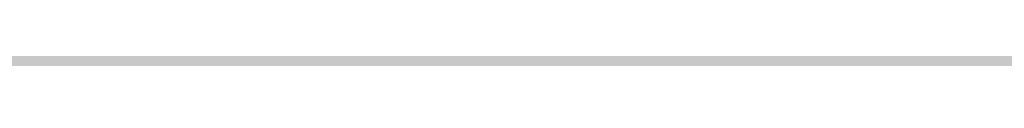
# Model space of a CAD drawing. Units: millimetres. Extents: x 0 to 2267, y 0 to 1823.
# Tile 97 of 256: x 1600.369 to 1605.705, y 1227.255 to 1227.263. Entities that reach past the tile are written whole.
import ezdxf

# ---------------------------------------------------------------- set-up
doc = ezdxf.new("R2010")
doc.units = ezdxf.units.MM
doc.header["$MEASUREMENT"] = 0
doc.layers.add('M-DIMS', color=2, linetype='Continuous', lineweight=25)
doc.layers.add('M-HATC', color=252, linetype='Continuous', lineweight=18)
doc.styles.get("Standard").update_dxf_attribs({"font": 'arial.ttf'})
doc.dimstyles.get("Standard").update_dxf_attribs({"dimtxt": 7, "dimasz": 4, "dimexe": 0.18, "dimexo": 0.0625, "dimgap": 0.09, "dimtad": 0, "dimdec": 0, "dimzin": 0, "dimdsep": 46, "dimtxsty": 'Standard', "dimcen": 0.09, "dimadec": 0, "dimazin": 0, "dimtfac": 1, "dimtdec": 0, "dimtofl": 0, "dimtmove": 0, "dimatfit": 3, "dimfxl": 1, "dimtolj": 1, "dimtzin": 0, "dimarcsym": 0})

# ---------------------------------------------------------------- blocks, each defined once
blk = doc.blocks.new('*D19')
at = {"layer": 'Defpoints', "color": 0, "transparency": 16777216}
for p in [(1605.3399, 1483.3044), (1445.5291, 1333.8851)]:
    blk.add_point(p, dxfattribs=at)
at = {"layer": 'M-DIMS', "color": 0, "lineweight": -2, "transparency": 16777216}
for p, q in [((1605.3399, 1483.2144), (1605.3399, 1483.3944)), ((1605.2499, 1483.3044), (1605.4299, 1483.3044)), ((1366.3244, 1259.8306), (1442.6072, 1331.1532))]:
    blk.add_line(p, q, dxfattribs=at)
at = {"layer": 'M-DIMS', "color": 0, "transparency": 16777216}
blk.add_solid([(1442.1519, 1331.6402), (1443.0625, 1330.6663), (1445.5291, 1333.8851)], dxfattribs=at)
at = {"layer": 'M-DIMS', "color": 0, "transparency": 16777216, "insert": (1349.6425, 1244.2335), "char_height": 7, "attachment_point": 5, "rotation": 43.0753}
blk.add_mtext('\\A1;2X R218.8', dxfattribs=at)

msp = doc.modelspace()

# ---------------------------------------------------------------- hatches: boundary and pattern name
at = {"layer": 'M-HATC'}
h = msp.add_hatch(color=256, dxfattribs=at)
h.dxf.hatch_style = 1
h.paths.add_polyline_path([(2055.771, 1603.062), (1381.0868, 1603.062), (1381.0868, 1598.062), (2055.771, 1598.062)])
h.paths.add_polyline_path([(2055.771, 1598.062), (1381.0868, 1598.062), (1381.0868, 1593.062), (2055.771, 1593.062)])
h.paths.add_polyline_path([(2051.3074, 1536.7609), (1385.5504, 1536.7609), (1385.5504, 1526.7609), (1387.5504, 1526.7609), (1388.5366, 1525.0528), (1385.3319, 1521.2335), (1385.3319, 1521.2226), (2050.2542, 1522.7491), (2048.3212, 1525.0528), (2049.3074, 1526.7609), (2051.3074, 1526.7609)])
edge = h.paths.add_edge_path()
edge.add_arc((1847.5345, 1379.1492), 135, 222.603061, 222.890851, ccw=False)
edge.add_line((1748.1663, 1287.7656), (1683.0921, 1287.7656))
edge.add_arc((1583.7239, 1379.1492), 135, 317.109149, 317.396939, ccw=False)
edge.add_arc((1678.9686, 1290.6707), 5, 222.8909, 317.1091, ccw=False)
edge.add_arc((1774.2133, 1379.1492), 135, 222.603061, 222.890851, ccw=False)
edge.add_line((1674.8451, 1287.7656), (1609.7709, 1287.7656))
edge.add_arc((1510.4027, 1379.1492), 135, 317.109149, 317.396939, ccw=False)
edge.add_arc((1605.6474, 1290.6707), 5, 222.8909, 317.1091, ccw=False)
edge.add_arc((1700.8921, 1379.1492), 135, 222.603061, 222.890851, ccw=False)
edge.add_line((1601.5239, 1287.7656), (1536.4497, 1287.7656))
edge.add_arc((1437.0815, 1379.1492), 135, 317.109149, 317.396939, ccw=False)
edge.add_arc((1532.3262, 1290.6707), 5, 222.8909, 317.1091, ccw=False)
edge.add_arc((1627.5709, 1379.1492), 135, 222.603061, 222.890851, ccw=False)
edge.add_line((1528.2027, 1287.7656), (1505.9289, 1287.7656))
edge.add_spline(control_points=[(1505.9289, 1287.7656), (1504.2622, 1287.7656), (1504.2622, 1282.7656), (1505.9289, 1282.7656)], knot_values=[0, 0, 0, 0, 5, 5, 5, 5], degree=3, periodic=0)
edge.add_line((1505.9289, 1282.7656), (1930.9289, 1282.7656))
edge.add_spline(control_points=[(1930.9289, 1282.7656), (1932.5956, 1282.7656), (1932.5956, 1287.7656), (1930.9289, 1287.7656)], knot_values=[0, 0, 0, 0, 5, 5, 5, 5], degree=3, periodic=0)
edge.add_line((1930.9289, 1287.7656), (1903.0557, 1287.7656))
edge.add_arc((1803.6875, 1379.1492), 135, 317.109149, 317.396939, ccw=False)
edge.add_arc((1898.9322, 1290.6707), 5, 222.8909, 317.1091, ccw=False)
edge.add_arc((1994.1769, 1379.1492), 135, 222.603061, 222.890851, ccw=False)
edge.add_line((1894.8087, 1287.7656), (1829.7345, 1287.7656))
edge.add_arc((1730.3663, 1379.1492), 135, 317.109149, 317.396939, ccw=False)
edge.add_arc((1825.611, 1290.6707), 5, 222.8909, 317.1091, ccw=False)
edge.add_arc((1920.8557, 1379.1492), 135, 222.603061, 222.890851, ccw=False)
edge.add_line((1821.4875, 1287.7656), (1756.4133, 1287.7656))
edge.add_arc((1657.0451, 1379.1492), 135, 317.109149, 317.396939, ccw=False)
edge.add_arc((1752.2898, 1290.6707), 5, 222.8909, 317.1091, ccw=False)
edge = h.paths.add_edge_path()
edge.add_spline(control_points=[(1843.4289, 1227.2475), (1845.0956, 1227.2475), (1845.0956, 1232.2475), (1843.4289, 1232.2475)], knot_values=[0, 0, 0, 0, 5, 5, 5, 5], degree=3, periodic=0)
edge.add_line((1843.4289, 1232.2475), (1593.4289, 1232.2475))
edge.add_spline(control_points=[(1593.4289, 1232.2475), (1591.7622, 1232.2475), (1591.7622, 1227.2475), (1593.4289, 1227.2475)], knot_values=[0, 0, 0, 0, 5, 5, 5, 5], degree=3, periodic=0)
edge.add_line((1593.4289, 1227.2475), (1843.4289, 1227.2475))
h.paths.add_polyline_path([(1905.9289, 1127.4171), (1530.9289, 1127.4171, 0.414214), (1520.9289, 1117.4171), (1530.9289, 1117.4171), (1915.9289, 1117.4171, 0.414214)])
edge = h.paths.add_edge_path()
edge.add_arc((1397.0858, 1498.4078), 12.7299, 90.78215, 190.87871, ccw=False)
edge.add_line((1396.912, 1511.1365), (1428.0097, 1511.3488))
edge.add_line((1428.0097, 1511.3488), (1433.0097, 1511.3488))
edge.add_line((1433.0097, 1511.3488), (1434.439, 1511.3488))
edge.add_arc((1419.474, 1498.0804), 20, 41.561, 74.08211)
edge.add_line((1424.9592, 1517.3135), (1399.9351, 1517.2561))
edge.add_spline(control_points=[(1399.9307, 1517.2561), (1399.884, 1517.2131), (1399.8328, 1517.1689), (1399.7774, 1517.1236)], knot_values=[11.567499, 11.567499, 11.567499, 11.567499, 11.814249, 11.814249, 11.814249, 11.814249], degree=3, periodic=0)
edge.add_spline(control_points=[(1399.6328, 1517.0099), (1399.5831, 1516.9721), (1399.5307, 1516.9338), (1399.4759, 1516.8947)], knot_values=[11.167718, 11.167718, 11.167718, 11.167718, 11.365188, 11.365188, 11.365188, 11.365188], degree=3, periodic=0)
edge.add_spline(control_points=[(1399.3398, 1516.8001), (1399.1514, 1516.6719), (1398.9384, 1516.5377), (1398.704, 1516.3994)], knot_values=[10.376405, 10.376405, 10.376405, 10.376405, 11.00994, 11.00994, 11.00994, 11.00994], degree=3, periodic=0)
edge.add_spline(control_points=[(1398.6572, 1516.3719), (1398.5789, 1516.326), (1398.4983, 1516.2797), (1398.4155, 1516.2331)], knot_values=[10.125175, 10.125175, 10.125175, 10.125175, 10.334406, 10.334406, 10.334406, 10.334406], degree=3, periodic=0)
edge.add_spline(control_points=[(1398.2642, 1516.1487), (1398.196, 1516.1111), (1398.1263, 1516.0732), (1398.0555, 1516.0351)], knot_values=[9.832246, 9.832246, 9.832246, 9.832246, 9.999658, 9.999658, 9.999658, 9.999658], degree=3, periodic=0)
edge.add_spline(control_points=[(1397.9987, 1516.0048), (1397.7312, 1515.8621), (1397.446, 1515.7171), (1397.1466, 1515.5714)], knot_values=[9.161808, 9.161808, 9.161808, 9.161808, 9.787769, 9.787769, 9.787769, 9.787769], degree=3, periodic=0)
edge.add_spline(control_points=[(1397.1466, 1515.5714), (1396.8418, 1515.423), (1396.5222, 1515.274), (1396.1914, 1515.1262)], knot_values=[8.524455, 8.524455, 8.524455, 8.524455, 9.161808, 9.161808, 9.161808, 9.161808], degree=3, periodic=0)
edge.add_spline(control_points=[(1396.0777, 1515.0756), (1395.9854, 1515.0348), (1395.8922, 1514.994), (1395.7983, 1514.9534)], knot_values=[8.275193, 8.275193, 8.275193, 8.275193, 8.451726, 8.451726, 8.451726, 8.451726], degree=3, periodic=0)
edge.add_spline(control_points=[(1395.6018, 1514.8691), (1395.4997, 1514.8257), (1395.3968, 1514.7824), (1395.2932, 1514.7394)], knot_values=[7.962917, 7.962917, 7.962917, 7.962917, 8.152764, 8.152764, 8.152764, 8.152764], degree=3, periodic=0)
edge.add_spline(control_points=[(1395.2116, 1514.7057), (1394.8278, 1514.5475), (1394.4345, 1514.3929), (1394.0364, 1514.2442)], knot_values=[7.21254, 7.21254, 7.21254, 7.21254, 7.913148, 7.913148, 7.913148, 7.913148], degree=3, periodic=0)
edge.add_spline(control_points=[(1394.0364, 1514.2442), (1393.7076, 1514.1214), (1393.3754, 1514.0027), (1393.0427, 1513.8895)], knot_values=[6.633733, 6.633733, 6.633733, 6.633733, 7.21254, 7.21254, 7.21254, 7.21254], degree=3, periodic=0)
edge.add_spline(control_points=[(1392.8214, 1513.815), (1392.7198, 1513.7812), (1392.6181, 1513.7479), (1392.5166, 1513.7152)], knot_values=[6.328796, 6.328796, 6.328796, 6.328796, 6.505493, 6.505493, 6.505493, 6.505493], degree=3, periodic=0)
edge.add_spline(control_points=[(1392.5166, 1513.7152), (1392.3187, 1513.6515), (1392.1212, 1513.59), (1391.9244, 1513.531)], knot_values=[5.984605, 5.984605, 5.984605, 5.984605, 6.328796, 6.328796, 6.328796, 6.328796], degree=3, periodic=0)
edge.add_spline(control_points=[(1391.7915, 1513.4915), (1391.3122, 1513.3501), (1390.8384, 1513.2239), (1390.3784, 1513.1171)], knot_values=[5.066697, 5.066697, 5.066697, 5.066697, 5.907055, 5.907055, 5.907055, 5.907055], degree=3, periodic=0)
edge.add_spline(control_points=[(1390.3784, 1513.1171), (1390.1797, 1513.071), (1389.9836, 1513.0284), (1389.7907, 1512.9899)], knot_values=[4.70367, 4.70367, 4.70367, 4.70367, 5.066695, 5.066695, 5.066695, 5.066695], degree=3, periodic=0)
edge.add_spline(control_points=[(1389.422, 1512.9204), (1389.2459, 1512.8892), (1389.0729, 1512.8617), (1388.9036, 1512.8381)], knot_values=[4.130571, 4.130571, 4.130571, 4.130571, 4.469816, 4.469816, 4.469816, 4.469816], degree=3, periodic=0)
edge.add_spline(control_points=[(1388.9036, 1512.8381), (1388.591, 1512.7946), (1388.2911, 1512.7644), (1388.0071, 1512.7494)], knot_values=[3.504031, 3.504031, 3.504031, 3.504031, 4.130571, 4.130571, 4.130571, 4.130571], degree=3, periodic=0)
edge.add_spline(control_points=[(1387.9356, 1512.7459), (1387.8538, 1512.7423), (1387.7733, 1512.74), (1387.6944, 1512.739)], knot_values=[3.268866, 3.268866, 3.268866, 3.268866, 3.451164, 3.451164, 3.451164, 3.451164], degree=3, periodic=0)
edge.add_spline(control_points=[(1387.3351, 1512.7443), (1387.2076, 1512.7499), (1387.0847, 1512.7597), (1386.967, 1512.7739)], knot_values=[2.670686, 2.670686, 2.670686, 2.670686, 2.984, 2.984, 2.984, 2.984], degree=3, periodic=0)
edge.add_spline(control_points=[(1386.8327, 1512.7922), (1386.8209, 1512.7941), (1386.8092, 1512.7959), (1386.7975, 1512.7979)], knot_values=[2.516981, 2.516981, 2.516981, 2.516981, 2.549528, 2.549528, 2.549528, 2.549528], degree=3, periodic=0)
edge.add_spline(control_points=[(1386.4526, 1512.8735), (1386.4257, 1512.881), (1386.3993, 1512.889), (1386.3733, 1512.8972)], knot_values=[2.095869, 2.095869, 2.095869, 2.095869, 2.17941, 2.17941, 2.17941, 2.17941], degree=3, periodic=0)
edge.add_spline(control_points=[(1386.0691, 1513.0189), (1386.0634, 1513.0217), (1386.0577, 1513.0246), (1386.052, 1513.0275)], knot_values=[1.72453, 1.72453, 1.72453, 1.72453, 1.745933, 1.745933, 1.745933, 1.745933], degree=3, periodic=0)
edge.add_arc((1399.474, 1498.0804), 20, 131.82432, 180)
edge.add_arc((1630.3336, 1505.5484), 250.9708, 181.705176, 236.427975)
edge.add_arc((1605.3399, 1483.3044), 218.7822, 238.660829, 243.34961)
edge.add_arc((1647.0911, 1510.3592), 262.8986, 183.129836, 237.853442, ccw=False)
h.paths.add_polyline_path([(1406.5369, 1391.9644, 0.149382), (1491.5506, 1296.4418, -0.129517)], flags=17)
edge = h.paths.add_edge_path()
edge.add_arc((2037.3838, 1498.0804), 20, 0, 48.26587)
edge.add_spline(control_points=[(2050.6973, 1513.0052), (2050.6512, 1512.9847), (2050.6034, 1512.9655), (2050.5539, 1512.9477)], knot_values=[1.835652, 1.835652, 1.835652, 1.835652, 2.000781, 2.000781, 2.000781, 2.000781], degree=3, periodic=0)
edge.add_spline(control_points=[(2050.4616, 1512.9166), (2050.479, 1512.9221), (2050.4963, 1512.9277), (2050.5133, 1512.9335)], knot_values=[2.045477, 2.045477, 2.045477, 2.045477, 2.101389, 2.101389, 2.101389, 2.101389], degree=3, periodic=0)
edge.add_spline(control_points=[(2050.129, 1512.8342), (2050.1984, 1512.8473), (2050.2657, 1512.8623), (2050.3308, 1512.8792)], knot_values=[2.237629, 2.237629, 2.237629, 2.237629, 2.435841, 2.435841, 2.435841, 2.435841], degree=3, periodic=0)
edge.add_spline(control_points=[(2050.0946, 1512.8278), (2050.1061, 1512.8299), (2050.1176, 1512.832), (2050.129, 1512.8342)], knot_values=[2.435841, 2.435841, 2.435841, 2.435841, 2.468321, 2.468321, 2.468321, 2.468321], degree=3, periodic=0)
edge.add_spline(control_points=[(2049.7843, 1512.7851), (2049.8552, 1512.7922), (2049.9243, 1512.8008), (2049.9917, 1512.8109)], knot_values=[2.563852, 2.563852, 2.563852, 2.563852, 2.748541, 2.748541, 2.748541, 2.748541], degree=3, periodic=0)
edge.add_spline(control_points=[(2049.4052, 1512.7617), (2049.5364, 1512.7653), (2049.6629, 1512.773), (2049.7843, 1512.7851)], knot_values=[2.748541, 2.748541, 2.748541, 2.748541, 3.064882, 3.064882, 3.064882, 3.064882], degree=3, periodic=0)
edge.add_spline(control_points=[(2049.1698, 1512.7597), (2049.2336, 1512.7591), (2049.2965, 1512.7594), (2049.3584, 1512.7606)], knot_values=[3.102309, 3.102309, 3.102309, 3.102309, 3.2503, 3.2503, 3.2503, 3.2503], degree=3, periodic=0)
edge.add_spline(control_points=[(2048.8573, 1512.7691), (2048.9638, 1512.7638), (2049.068, 1512.7606), (2049.1698, 1512.7597)], knot_values=[3.2503, 3.2503, 3.2503, 3.2503, 3.486069, 3.486069, 3.486069, 3.486069], degree=3, periodic=0)
edge.add_spline(control_points=[(2048.6924, 1512.7789), (2048.3729, 1512.8009), (2048.0345, 1512.8411), (2047.6817, 1512.897)], knot_values=[3.606429, 3.606429, 3.606429, 3.606429, 4.2989, 4.2989, 4.2989, 4.2989], degree=3, periodic=0)
edge.add_spline(control_points=[(2047.6817, 1512.897), (2047.5458, 1512.9185), (2047.4077, 1512.9424), (2047.2678, 1512.9685)], knot_values=[4.2989, 4.2989, 4.2989, 4.2989, 4.565769, 4.565769, 4.565769, 4.565769], degree=3, periodic=0)
edge.add_spline(control_points=[(2047.2678, 1512.9685), (2047.1449, 1512.9914), (2047.0207, 1513.016), (2046.8951, 1513.0422)], knot_values=[4.565769, 4.565769, 4.565769, 4.565769, 4.799971, 4.799971, 4.799971, 4.799971], degree=3, periodic=0)
edge.add_spline(control_points=[(2046.8951, 1513.0422), (2046.5286, 1513.1188), (2046.1513, 1513.209), (2045.7676, 1513.3107)], knot_values=[4.799971, 4.799971, 4.799971, 4.799971, 5.483718, 5.483718, 5.483718, 5.483718], degree=3, periodic=0)
edge.add_spline(control_points=[(2045.7676, 1513.3107), (2045.3724, 1513.4154), (2044.9704, 1513.5322), (2044.5662, 1513.6588)], knot_values=[5.483718, 5.483718, 5.483718, 5.483718, 6.187866, 6.187866, 6.187866, 6.187866], degree=3, periodic=0)
edge.add_spline(control_points=[(2044.5662, 1513.6588), (2044.4149, 1513.7061), (2044.2633, 1513.7549), (2044.1116, 1513.8048)], knot_values=[6.187866, 6.187866, 6.187866, 6.187866, 6.451551, 6.451551, 6.451551, 6.451551], degree=3, periodic=0)
edge.add_spline(control_points=[(2044.1116, 1513.8048), (2043.9967, 1513.8427), (2043.8817, 1513.8813), (2043.7668, 1513.9205)], knot_values=[6.451551, 6.451551, 6.451551, 6.451551, 6.651434, 6.651434, 6.651434, 6.651434], degree=3, periodic=0)
edge.add_spline(control_points=[(2043.7668, 1513.9205), (2043.3716, 1514.0554), (2042.9774, 1514.1979), (2042.5886, 1514.3458)], knot_values=[6.651434, 6.651434, 6.651434, 6.651434, 7.338879, 7.338879, 7.338879, 7.338879], degree=3, periodic=0)
edge.add_spline(control_points=[(2042.5886, 1514.3458), (2042.1643, 1514.5071), (2041.7465, 1514.6749), (2041.3409, 1514.846)], knot_values=[7.338879, 7.338879, 7.338879, 7.338879, 8.089209, 8.089209, 8.089209, 8.089209], degree=3, periodic=0)
edge.add_spline(control_points=[(2041.3409, 1514.846), (2041.1028, 1514.9465), (2040.869, 1515.0481), (2040.6405, 1515.1502)], knot_values=[8.089209, 8.089209, 8.089209, 8.089209, 8.529587, 8.529587, 8.529587, 8.529587], degree=3, periodic=0)
edge.add_spline(control_points=[(2040.51, 1515.2089), (2040.0824, 1515.4022), (2039.6747, 1515.5971), (2039.295, 1515.7894)], knot_values=[8.613818, 8.613818, 8.613818, 8.613818, 9.44571, 9.44571, 9.44571, 9.44571], degree=3, periodic=0)
edge.add_spline(control_points=[(2039.295, 1515.7894), (2039.0618, 1515.9075), (2038.8391, 1516.0246), (2038.6288, 1516.1398)], knot_values=[9.44571, 9.44571, 9.44571, 9.44571, 9.956404, 9.956404, 9.956404, 9.956404], degree=3, periodic=0)
edge.add_spline(control_points=[(2038.6288, 1516.1398), (2038.5187, 1516.2001), (2038.4121, 1516.2598), (2038.309, 1516.3189)], knot_values=[9.956404, 9.956404, 9.956404, 9.956404, 10.223542, 10.223542, 10.223542, 10.223542], degree=3, periodic=0)
edge.add_spline(control_points=[(2038.309, 1516.3189), (2038.2138, 1516.3735), (2038.1216, 1516.4276), (2038.0328, 1516.481)], knot_values=[10.223542, 10.223542, 10.223542, 10.223542, 10.47051, 10.47051, 10.47051, 10.47051], degree=3, periodic=0)
edge.add_spline(control_points=[(2038.0328, 1516.481), (2037.7855, 1516.6296), (2037.5639, 1516.773), (2037.3722, 1516.909)], knot_values=[10.47051, 10.47051, 10.47051, 10.47051, 11.15767, 11.15767, 11.15767, 11.15767], degree=3, periodic=0)
edge.add_spline(control_points=[(2037.3722, 1516.909), (2037.2789, 1516.9752), (2037.1927, 1517.0396), (2037.1142, 1517.102)], knot_values=[11.15767, 11.15767, 11.15767, 11.15767, 11.49227, 11.49227, 11.49227, 11.49227], degree=3, periodic=0)
edge.add_spline(control_points=[(2036.8564, 1517.3259), (2036.9148, 1517.2692), (2036.9814, 1517.2103), (2037.0557, 1517.1492)], knot_values=[11.577341, 11.577341, 11.577341, 11.577341, 11.91035, 11.91035, 11.91035, 11.91035], degree=3, periodic=0)
edge.add_spline(control_points=[(2036.8074, 1517.3748), (2036.823, 1517.3587), (2036.8393, 1517.3424), (2036.8564, 1517.3259)], knot_values=[11.91035, 11.91035, 11.91035, 11.91035, 12.007402, 12.007402, 12.007402, 12.007402], degree=3, periodic=0)
edge.add_spline(control_points=[(2036.7017, 1517.494), (2036.7104, 1517.483), (2036.7196, 1517.4719), (2036.7291, 1517.4606)], knot_values=[12.184155, 12.184155, 12.184155, 12.184155, 12.255409, 12.255409, 12.255409, 12.255409], degree=3, periodic=0)
edge.add_spline(control_points=[(2036.6159, 1517.6205), (2036.62, 1517.613), (2036.6243, 1517.6055), (2036.6289, 1517.5979)], knot_values=[12.487913, 12.487913, 12.487913, 12.487913, 12.541035, 12.541035, 12.541035, 12.541035], degree=3, periodic=0)
edge.add_spline(control_points=[(2036.5635, 1517.786), (2036.5637, 1517.7794), (2036.5642, 1517.7726), (2036.565, 1517.7658)], knot_values=[12.911761, 12.911761, 12.911761, 12.911761, 12.968286, 12.968286, 12.968286, 12.968286], degree=3, periodic=0)
edge.add_spline(control_points=[(2036.6166, 1517.9304), (2036.6125, 1517.9259), (2036.6086, 1517.9212), (2036.6049, 1517.9165)], knot_values=[13.382527, 13.382527, 13.382527, 13.382527, 13.433791, 13.433791, 13.433791, 13.433791], degree=3, periodic=0)
edge.add_spline(control_points=[(2036.749, 1518.017), (2036.7361, 1518.0116), (2036.7239, 1518.006), (2036.7124, 1518.0002)], knot_values=[13.726299, 13.726299, 13.726299, 13.726299, 13.809928, 13.809928, 13.809928, 13.809928], degree=3, periodic=0)
edge.add_spline(control_points=[(2036.8604, 1518.0528), (2036.8386, 1518.0474), (2036.8181, 1518.0416), (2036.7988, 1518.0353)], knot_values=[13.910887, 13.910887, 13.910887, 13.910887, 14.02153, 14.02153, 14.02153, 14.02153], degree=3, periodic=0)
edge.add_line((2036.9639, 1518.0804), (2032.3838, 1518.0804))
edge.add_line((2032.3838, 1518.0804), (2027.3838, 1518.0804))
edge.add_line((2027.3838, 1518.0804), (2022.3838, 1518.0804))
edge.add_line((2022.3838, 1518.0804), (2017.3838, 1518.0804))
edge.add_arc((2017.3838, 1498.0804), 20, 90, 138.439)
edge.add_line((2002.4188, 1511.3488), (2003.8481, 1511.3488))
edge.add_line((2003.8481, 1511.3488), (2008.8481, 1511.3488))
edge.add_line((2008.8481, 1511.3488), (2039.772, 1511.1377))
edge.add_arc((2039.772, 1498.4078), 12.7299, -10.87871, 90, ccw=False)
edge.add_arc((1789.7668, 1510.3592), 262.8986, 302.146558, 356.870164, ccw=False)
edge.add_arc((1831.5179, 1483.3044), 218.7822, 296.65039, 301.339171)
edge.add_arc((1806.5242, 1505.5484), 250.9708, 303.572025, 358.294824)
h.paths.add_polyline_path([(2030.321, 1391.9644, -0.129517), (1945.3072, 1296.4418, 0.149382)], flags=17)
edge = h.paths.add_edge_path()
edge.add_spline(control_points=[(2037.2464, 1518.0821), (2037.2898, 1518.081), (2037.3355, 1518.0804), (2037.3838, 1518.0804)], knot_values=[0.000012, 0.000012, 0.000012, 0.000012, 0.144754, 0.144754, 0.144754, 0.144754], degree=3, periodic=0)
edge.add_line((2037.3357, 1518.0804), (2037.0096, 1518.0804))
edge.add_spline(control_points=[(2037.0096, 1518.0804), (2036.9822, 1518.0768), (2036.956, 1518.0727), (2036.9312, 1518.0681)], knot_values=[14.13465, 14.13465, 14.13465, 14.13465, 14.247197, 14.247197, 14.247197, 14.247197], degree=3, periodic=0)
edge.add_spline(control_points=[(2036.9312, 1518.0681), (2036.9276, 1518.0674), (2036.9241, 1518.0667), (2036.9205, 1518.0661)], knot_values=[14.118315, 14.118315, 14.118315, 14.118315, 14.13465, 14.13465, 14.13465, 14.13465], degree=3, periodic=0)
edge.add_spline(control_points=[(2036.9205, 1518.0661), (2036.9118, 1518.0644), (2036.9032, 1518.0626), (2036.8948, 1518.0608)], knot_values=[14.078086, 14.078086, 14.078086, 14.078086, 14.118315, 14.118315, 14.118315, 14.118315], degree=3, periodic=0)
edge.add_spline(control_points=[(2036.8948, 1518.0608), (2036.883, 1518.0583), (2036.8716, 1518.0556), (2036.8604, 1518.0528)], knot_values=[14.02153, 14.02153, 14.02153, 14.02153, 14.078086, 14.078086, 14.078086, 14.078086], degree=3, periodic=0)
edge.add_spline(control_points=[(2036.8604, 1518.0528), (2036.8386, 1518.0474), (2036.8181, 1518.0416), (2036.7988, 1518.0353)], knot_values=[13.910887, 13.910887, 13.910887, 13.910887, 14.02153, 14.02153, 14.02153, 14.02153], degree=3, periodic=0)
edge.add_spline(control_points=[(2036.7988, 1518.0353), (2036.7981, 1518.035), (2036.7974, 1518.0348), (2036.7967, 1518.0346)], knot_values=[13.906906, 13.906906, 13.906906, 13.906906, 13.910887, 13.910887, 13.910887, 13.910887], degree=3, periodic=0)
edge.add_spline(control_points=[(2036.7967, 1518.0346), (2036.7882, 1518.0318), (2036.7799, 1518.0289), (2036.7719, 1518.0259)], knot_values=[13.857826, 13.857826, 13.857826, 13.857826, 13.906906, 13.906906, 13.906906, 13.906906], degree=3, periodic=0)
edge.add_spline(control_points=[(2036.7719, 1518.0259), (2036.764, 1518.023), (2036.7564, 1518.02), (2036.749, 1518.017)], knot_values=[13.809928, 13.809928, 13.809928, 13.809928, 13.857826, 13.857826, 13.857826, 13.857826], degree=3, periodic=0)
edge.add_spline(control_points=[(2036.749, 1518.017), (2036.7361, 1518.0116), (2036.7239, 1518.006), (2036.7124, 1518.0002)], knot_values=[13.726299, 13.726299, 13.726299, 13.726299, 13.809928, 13.809928, 13.809928, 13.809928], degree=3, periodic=0)
edge.add_spline(control_points=[(2036.7124, 1518.0002), (2036.7121, 1518), (2036.7118, 1517.9999), (2036.7115, 1517.9997)], knot_values=[13.723993, 13.723993, 13.723993, 13.723993, 13.726299, 13.726299, 13.726299, 13.726299], degree=3, periodic=0)
edge.add_spline(control_points=[(2036.7115, 1517.9997), (2036.7063, 1517.9971), (2036.7013, 1517.9944), (2036.6965, 1517.9917)], knot_values=[13.686536, 13.686536, 13.686536, 13.686536, 13.723993, 13.723993, 13.723993, 13.723993], degree=3, periodic=0)
edge.add_spline(control_points=[(2036.6965, 1517.9917), (2036.6919, 1517.9891), (2036.6874, 1517.9865), (2036.6831, 1517.9839)], knot_values=[13.651251, 13.651251, 13.651251, 13.651251, 13.686536, 13.686536, 13.686536, 13.686536], degree=3, periodic=0)
edge.add_spline(control_points=[(2036.6831, 1517.9839), (2036.6764, 1517.9798), (2036.67, 1517.9757), (2036.6639, 1517.9714)], knot_values=[13.596804, 13.596804, 13.596804, 13.596804, 13.651251, 13.651251, 13.651251, 13.651251], degree=3, periodic=0)
edge.add_spline(control_points=[(2036.6639, 1517.9714), (2036.6636, 1517.9712), (2036.6633, 1517.9709), (2036.6629, 1517.9707)], knot_values=[13.593956, 13.593956, 13.593956, 13.593956, 13.596804, 13.596804, 13.596804, 13.596804], degree=3, periodic=0)
edge.add_spline(control_points=[(2036.6629, 1517.9707), (2036.6603, 1517.9689), (2036.6577, 1517.967), (2036.6552, 1517.9651)], knot_values=[13.570322, 13.570322, 13.570322, 13.570322, 13.593956, 13.593956, 13.593956, 13.593956], degree=3, periodic=0)
edge.add_spline(control_points=[(2036.6552, 1517.9651), (2036.6525, 1517.9631), (2036.6499, 1517.9611), (2036.6474, 1517.9591)], knot_values=[13.545477, 13.545477, 13.545477, 13.545477, 13.570322, 13.570322, 13.570322, 13.570322], degree=3, periodic=0)
edge.add_spline(control_points=[(2036.6474, 1517.9591), (2036.6472, 1517.9589), (2036.6471, 1517.9588), (2036.6469, 1517.9587)], knot_values=[13.543931, 13.543931, 13.543931, 13.543931, 13.545477, 13.545477, 13.545477, 13.545477], degree=3, periodic=0)
edge.add_spline(control_points=[(2036.6469, 1517.9587), (2036.6412, 1517.9541), (2036.6358, 1517.9494), (2036.6307, 1517.9447)], knot_values=[13.488237, 13.488237, 13.488237, 13.488237, 13.543931, 13.543931, 13.543931, 13.543931], degree=3, periodic=0)
edge.add_spline(control_points=[(2036.6307, 1517.9447), (2036.6282, 1517.9423), (2036.6257, 1517.9399), (2036.6233, 1517.9374)], knot_values=[13.460307, 13.460307, 13.460307, 13.460307, 13.488237, 13.488237, 13.488237, 13.488237], degree=3, periodic=0)
edge.add_spline(control_points=[(2036.6233, 1517.9374), (2036.6215, 1517.9356), (2036.6198, 1517.9338), (2036.6181, 1517.932)], knot_values=[13.439712, 13.439712, 13.439712, 13.439712, 13.460307, 13.460307, 13.460307, 13.460307], degree=3, periodic=0)
edge.add_spline(control_points=[(2036.6181, 1517.932), (2036.6176, 1517.9315), (2036.6171, 1517.9309), (2036.6166, 1517.9304)], knot_values=[13.433791, 13.433791, 13.433791, 13.433791, 13.439712, 13.439712, 13.439712, 13.439712], degree=3, periodic=0)
edge.add_spline(control_points=[(2036.6166, 1517.9304), (2036.6125, 1517.9259), (2036.6086, 1517.9212), (2036.6049, 1517.9165)], knot_values=[13.382527, 13.382527, 13.382527, 13.382527, 13.433791, 13.433791, 13.433791, 13.433791], degree=3, periodic=0)
edge.add_spline(control_points=[(2036.6049, 1517.9165), (2036.6026, 1517.9135), (2036.6004, 1517.9104), (2036.5982, 1517.9074)], knot_values=[13.350017, 13.350017, 13.350017, 13.350017, 13.382527, 13.382527, 13.382527, 13.382527], degree=3, periodic=0)
edge.add_spline(control_points=[(2036.5982, 1517.9074), (2036.5972, 1517.9059), (2036.5962, 1517.9043), (2036.5952, 1517.9028)], knot_values=[13.333922, 13.333922, 13.333922, 13.333922, 13.350017, 13.350017, 13.350017, 13.350017], degree=3, periodic=0)
edge.add_spline(control_points=[(2036.5952, 1517.9028), (2036.5945, 1517.9018), (2036.5939, 1517.9009), (2036.5933, 1517.8999)], knot_values=[13.323828, 13.323828, 13.323828, 13.323828, 13.333922, 13.333922, 13.333922, 13.333922], degree=3, periodic=0)
edge.add_spline(control_points=[(2036.5933, 1517.8999), (2036.5905, 1517.8955), (2036.5879, 1517.8909), (2036.5855, 1517.8864)], knot_values=[13.277545, 13.277545, 13.277545, 13.277545, 13.323828, 13.323828, 13.323828, 13.323828], degree=3, periodic=0)
edge.add_spline(control_points=[(2036.5855, 1517.8864), (2036.5836, 1517.8827), (2036.5817, 1517.8789), (2036.5801, 1517.8751)], knot_values=[13.240119, 13.240119, 13.240119, 13.240119, 13.277545, 13.277545, 13.277545, 13.277545], degree=3, periodic=0)
edge.add_spline(control_points=[(2036.5801, 1517.8751), (2036.5795, 1517.8739), (2036.579, 1517.8727), (2036.5785, 1517.8715)], knot_values=[13.228211, 13.228211, 13.228211, 13.228211, 13.240119, 13.240119, 13.240119, 13.240119], degree=3, periodic=0)
edge.add_spline(control_points=[(2036.5785, 1517.8715), (2036.578, 1517.8702), (2036.5774, 1517.869), (2036.5769, 1517.8677)], knot_values=[13.215717, 13.215717, 13.215717, 13.215717, 13.228211, 13.228211, 13.228211, 13.228211], degree=3, periodic=0)
edge.add_spline(control_points=[(2036.5769, 1517.8677), (2036.5755, 1517.864), (2036.5741, 1517.8603), (2036.5729, 1517.8565)], knot_values=[13.179847, 13.179847, 13.179847, 13.179847, 13.215717, 13.215717, 13.215717, 13.215717], degree=3, periodic=0)
edge.add_spline(control_points=[(2036.5729, 1517.8565), (2036.5713, 1517.8515), (2036.5699, 1517.8464), (2036.5687, 1517.8413)], knot_values=[13.132017, 13.132017, 13.132017, 13.132017, 13.179847, 13.179847, 13.179847, 13.179847], degree=3, periodic=0)
edge.add_spline(control_points=[(2036.5687, 1517.8413), (2036.5684, 1517.8402), (2036.5682, 1517.8392), (2036.568, 1517.8382)], knot_values=[13.122482, 13.122482, 13.122482, 13.122482, 13.132017, 13.132017, 13.132017, 13.132017], degree=3, periodic=0)
edge.add_spline(control_points=[(2036.568, 1517.8382), (2036.5676, 1517.8363), (2036.5672, 1517.8345), (2036.5669, 1517.8327)], knot_values=[13.105592, 13.105592, 13.105592, 13.105592, 13.122482, 13.122482, 13.122482, 13.122482], degree=3, periodic=0)
edge.add_spline(control_points=[(2036.5669, 1517.8327), (2036.5662, 1517.8292), (2036.5657, 1517.8257), (2036.5652, 1517.8222)], knot_values=[13.074063, 13.074063, 13.074063, 13.074063, 13.105592, 13.105592, 13.105592, 13.105592], degree=3, periodic=0)
edge.add_spline(control_points=[(2036.5652, 1517.8222), (2036.5652, 1517.8222), (2036.5652, 1517.8222), (2036.5652, 1517.8222)], knot_values=[13.074043, 13.074043, 13.074043, 13.074043, 13.074063, 13.074063, 13.074063, 13.074063], degree=3, periodic=0)
edge.add_spline(control_points=[(2036.5652, 1517.8222), (2036.5644, 1517.8164), (2036.5639, 1517.8106), (2036.5636, 1517.8046)], knot_values=[13.021884, 13.021884, 13.021884, 13.021884, 13.074043, 13.074043, 13.074043, 13.074043], degree=3, periodic=0)
edge.add_spline(control_points=[(2036.5636, 1517.8046), (2036.5636, 1517.804), (2036.5636, 1517.8034), (2036.5635, 1517.8028)], knot_values=[13.01674, 13.01674, 13.01674, 13.01674, 13.021884, 13.021884, 13.021884, 13.021884], degree=3, periodic=0)
edge.add_spline(control_points=[(2036.5635, 1517.8028), (2036.5634, 1517.8005), (2036.5634, 1517.7982), (2036.5634, 1517.7958)], knot_values=[12.996438, 12.996438, 12.996438, 12.996438, 13.01674, 13.01674, 13.01674, 13.01674], degree=3, periodic=0)
edge.add_spline(control_points=[(2036.5634, 1517.7958), (2036.5633, 1517.7926), (2036.5634, 1517.7893), (2036.5635, 1517.786)], knot_values=[12.968286, 12.968286, 12.968286, 12.968286, 12.996438, 12.996438, 12.996438, 12.996438], degree=3, periodic=0)
edge.add_spline(control_points=[(2036.5635, 1517.786), (2036.5637, 1517.7794), (2036.5642, 1517.7726), (2036.565, 1517.7658)], knot_values=[12.911761, 12.911761, 12.911761, 12.911761, 12.968286, 12.968286, 12.968286, 12.968286], degree=3, periodic=0)
edge.add_spline(control_points=[(2036.565, 1517.7658), (2036.565, 1517.7657), (2036.565, 1517.7656), (2036.565, 1517.7656)], knot_values=[12.911017, 12.911017, 12.911017, 12.911017, 12.911761, 12.911761, 12.911761, 12.911761], degree=3, periodic=0)
edge.add_spline(control_points=[(2036.565, 1517.7656), (2036.5654, 1517.7625), (2036.5658, 1517.7593), (2036.5663, 1517.7562)], knot_values=[12.88528, 12.88528, 12.88528, 12.88528, 12.911017, 12.911017, 12.911017, 12.911017], degree=3, periodic=0)
edge.add_spline(control_points=[(2036.5663, 1517.7562), (2036.5667, 1517.7534), (2036.5672, 1517.7506), (2036.5677, 1517.7478)], knot_values=[12.862519, 12.862519, 12.862519, 12.862519, 12.88528, 12.88528, 12.88528, 12.88528], degree=3, periodic=0)
edge.add_spline(control_points=[(2036.5677, 1517.7478), (2036.5678, 1517.7474), (2036.5679, 1517.7469), (2036.568, 1517.7465)], knot_values=[12.858885, 12.858885, 12.858885, 12.858885, 12.862519, 12.862519, 12.862519, 12.862519], degree=3, periodic=0)
edge.add_spline(control_points=[(2036.568, 1517.7465), (2036.5692, 1517.7399), (2036.5707, 1517.7332), (2036.5724, 1517.7264)], knot_values=[12.8053, 12.8053, 12.8053, 12.8053, 12.858885, 12.858885, 12.858885, 12.858885], degree=3, periodic=0)
edge.add_spline(control_points=[(2036.5724, 1517.7264), (2036.5734, 1517.7226), (2036.5745, 1517.7187), (2036.5756, 1517.7149)], knot_values=[12.775176, 12.775176, 12.775176, 12.775176, 12.8053, 12.8053, 12.8053, 12.8053], degree=3, periodic=0)
edge.add_spline(control_points=[(2036.5756, 1517.7149), (2036.5763, 1517.7125), (2036.577, 1517.7102), (2036.5778, 1517.7078)], knot_values=[12.756759, 12.756759, 12.756759, 12.756759, 12.775176, 12.775176, 12.775176, 12.775176], degree=3, periodic=0)
edge.add_spline(control_points=[(2036.5778, 1517.7078), (2036.5781, 1517.7067), (2036.5784, 1517.7057), (2036.5787, 1517.7047)], knot_values=[12.748742, 12.748742, 12.748742, 12.748742, 12.756759, 12.756759, 12.756759, 12.756759], degree=3, periodic=0)
edge.add_spline(control_points=[(2036.5787, 1517.7047), (2036.5808, 1517.6983), (2036.5831, 1517.6919), (2036.5856, 1517.6854)], knot_values=[12.69959, 12.69959, 12.69959, 12.69959, 12.748742, 12.748742, 12.748742, 12.748742], degree=3, periodic=0)
edge.add_spline(control_points=[(2036.5856, 1517.6854), (2036.5876, 1517.68), (2036.5898, 1517.6746), (2036.5921, 1517.6692)], knot_values=[12.659038, 12.659038, 12.659038, 12.659038, 12.69959, 12.69959, 12.69959, 12.69959], degree=3, periodic=0)
edge.add_spline(control_points=[(2036.5921, 1517.6692), (2036.594, 1517.6648), (2036.5959, 1517.6605), (2036.5979, 1517.6561)], knot_values=[12.626806, 12.626806, 12.626806, 12.626806, 12.659038, 12.659038, 12.659038, 12.659038], degree=3, periodic=0)
edge.add_spline(control_points=[(2036.5979, 1517.6561), (2036.5984, 1517.6551), (2036.5989, 1517.6541), (2036.5993, 1517.6531)], knot_values=[12.619394, 12.619394, 12.619394, 12.619394, 12.626806, 12.626806, 12.626806, 12.626806], degree=3, periodic=0)
edge.add_spline(control_points=[(2036.5993, 1517.6531), (2036.6043, 1517.6424), (2036.6099, 1517.6315), (2036.6159, 1517.6205)], knot_values=[12.541039, 12.541039, 12.541039, 12.541039, 12.619394, 12.619394, 12.619394, 12.619394], degree=3, periodic=0)
edge.add_spline(control_points=[(2036.6159, 1517.6205), (2036.6159, 1517.6205), (2036.6159, 1517.6205), (2036.6159, 1517.6205)], knot_values=[12.541035, 12.541035, 12.541035, 12.541035, 12.541039, 12.541039, 12.541039, 12.541039], degree=3, periodic=0)
edge.add_spline(control_points=[(2036.6159, 1517.6205), (2036.62, 1517.613), (2036.6243, 1517.6055), (2036.6289, 1517.5979)], knot_values=[12.487913, 12.487913, 12.487913, 12.487913, 12.541035, 12.541035, 12.541035, 12.541035], degree=3, periodic=0)
edge.add_spline(control_points=[(2036.6289, 1517.5979), (2036.6326, 1517.5916), (2036.6365, 1517.5853), (2036.6406, 1517.5789)], knot_values=[12.443982, 12.443982, 12.443982, 12.443982, 12.487913, 12.487913, 12.487913, 12.487913], degree=3, periodic=0)
edge.add_spline(control_points=[(2036.6406, 1517.5789), (2036.6414, 1517.5776), (2036.6423, 1517.5763), (2036.6431, 1517.5749)], knot_values=[12.434996, 12.434996, 12.434996, 12.434996, 12.443982, 12.443982, 12.443982, 12.443982], degree=3, periodic=0)
edge.add_spline(control_points=[(2036.6431, 1517.5749), (2036.6531, 1517.5596), (2036.6639, 1517.5439), (2036.6756, 1517.528)], knot_values=[12.329647, 12.329647, 12.329647, 12.329647, 12.434996, 12.434996, 12.434996, 12.434996], degree=3, periodic=0)
edge.add_spline(control_points=[(2036.6756, 1517.528), (2036.6839, 1517.5168), (2036.6925, 1517.5055), (2036.7017, 1517.494)], knot_values=[12.255409, 12.255409, 12.255409, 12.255409, 12.329647, 12.329647, 12.329647, 12.329647], degree=3, periodic=0)
edge.add_spline(control_points=[(2036.7017, 1517.494), (2036.7104, 1517.483), (2036.7196, 1517.4719), (2036.7291, 1517.4606)], knot_values=[12.184155, 12.184155, 12.184155, 12.184155, 12.255409, 12.255409, 12.255409, 12.255409], degree=3, periodic=0)
edge.add_spline(control_points=[(2036.7291, 1517.4606), (2036.7436, 1517.4435), (2036.759, 1517.4262), (2036.7753, 1517.4085)], knot_values=[12.075961, 12.075961, 12.075961, 12.075961, 12.184155, 12.184155, 12.184155, 12.184155], degree=3, periodic=0)
edge.add_spline(control_points=[(2036.7753, 1517.4085), (2036.7763, 1517.4075), (2036.7773, 1517.4064), (2036.7783, 1517.4054)], knot_values=[12.069502, 12.069502, 12.069502, 12.069502, 12.075961, 12.075961, 12.075961, 12.075961], degree=3, periodic=0)
edge.add_spline(control_points=[(2036.7783, 1517.4054), (2036.7877, 1517.3953), (2036.7974, 1517.385), (2036.8074, 1517.3748)], knot_values=[12.007402, 12.007402, 12.007402, 12.007402, 12.069502, 12.069502, 12.069502, 12.069502], degree=3, periodic=0)
edge.add_spline(control_points=[(2036.8074, 1517.3748), (2036.823, 1517.3587), (2036.8393, 1517.3424), (2036.8564, 1517.3259)], knot_values=[11.91035, 11.91035, 11.91035, 11.91035, 12.007402, 12.007402, 12.007402, 12.007402], degree=3, periodic=0)
edge.add_spline(control_points=[(2036.8564, 1517.3259), (2036.9148, 1517.2692), (2036.9814, 1517.2103), (2037.0557, 1517.1492)], knot_values=[11.577341, 11.577341, 11.577341, 11.577341, 11.91035, 11.91035, 11.91035, 11.91035], degree=3, periodic=0)
edge.add_spline(control_points=[(2037.0557, 1517.1492), (2037.0747, 1517.1336), (2037.0942, 1517.1179), (2037.1142, 1517.102)], knot_values=[11.49227, 11.49227, 11.49227, 11.49227, 11.577341, 11.577341, 11.577341, 11.577341], degree=3, periodic=0)
edge.add_spline(control_points=[(2037.1142, 1517.102), (2037.1927, 1517.0396), (2037.2789, 1516.9752), (2037.3722, 1516.909)], knot_values=[11.15767, 11.15767, 11.15767, 11.15767, 11.49227, 11.49227, 11.49227, 11.49227], degree=3, periodic=0)
edge.add_spline(control_points=[(2037.3722, 1516.909), (2037.5639, 1516.773), (2037.7855, 1516.6296), (2038.0328, 1516.481)], knot_values=[10.47051, 10.47051, 10.47051, 10.47051, 11.15767, 11.15767, 11.15767, 11.15767], degree=3, periodic=0)
edge.add_spline(control_points=[(2038.0328, 1516.481), (2038.1216, 1516.4276), (2038.2138, 1516.3735), (2038.309, 1516.3189)], knot_values=[10.223542, 10.223542, 10.223542, 10.223542, 10.47051, 10.47051, 10.47051, 10.47051], degree=3, periodic=0)
edge.add_spline(control_points=[(2038.309, 1516.3189), (2038.4121, 1516.2598), (2038.5187, 1516.2001), (2038.6288, 1516.1398)], knot_values=[9.956404, 9.956404, 9.956404, 9.956404, 10.223542, 10.223542, 10.223542, 10.223542], degree=3, periodic=0)
edge.add_spline(control_points=[(2038.6288, 1516.1398), (2038.8391, 1516.0246), (2039.0618, 1515.9075), (2039.295, 1515.7894)], knot_values=[9.44571, 9.44571, 9.44571, 9.44571, 9.956404, 9.956404, 9.956404, 9.956404], degree=3, periodic=0)
edge.add_spline(control_points=[(2039.295, 1515.7894), (2039.6747, 1515.5971), (2040.0824, 1515.4022), (2040.51, 1515.2089)], knot_values=[8.613818, 8.613818, 8.613818, 8.613818, 9.44571, 9.44571, 9.44571, 9.44571], degree=3, periodic=0)
edge.add_spline(control_points=[(2040.51, 1515.2089), (2040.5533, 1515.1893), (2040.5968, 1515.1697), (2040.6405, 1515.1502)], knot_values=[8.529587, 8.529587, 8.529587, 8.529587, 8.613818, 8.613818, 8.613818, 8.613818], degree=3, periodic=0)
edge.add_spline(control_points=[(2040.6405, 1515.1502), (2040.869, 1515.0481), (2041.1028, 1514.9465), (2041.3409, 1514.846)], knot_values=[8.089209, 8.089209, 8.089209, 8.089209, 8.529587, 8.529587, 8.529587, 8.529587], degree=3, periodic=0)
edge.add_spline(control_points=[(2041.3409, 1514.846), (2041.7465, 1514.6749), (2042.1643, 1514.5071), (2042.5886, 1514.3458)], knot_values=[7.338879, 7.338879, 7.338879, 7.338879, 8.089209, 8.089209, 8.089209, 8.089209], degree=3, periodic=0)
edge.add_spline(control_points=[(2042.5886, 1514.3458), (2042.9774, 1514.1979), (2043.3716, 1514.0554), (2043.7668, 1513.9205)], knot_values=[6.651434, 6.651434, 6.651434, 6.651434, 7.338879, 7.338879, 7.338879, 7.338879], degree=3, periodic=0)
edge.add_spline(control_points=[(2043.7668, 1513.9205), (2043.8817, 1513.8813), (2043.9967, 1513.8427), (2044.1116, 1513.8048)], knot_values=[6.451551, 6.451551, 6.451551, 6.451551, 6.651434, 6.651434, 6.651434, 6.651434], degree=3, periodic=0)
edge.add_spline(control_points=[(2044.1116, 1513.8048), (2044.2633, 1513.7549), (2044.4149, 1513.7061), (2044.5662, 1513.6588)], knot_values=[6.187866, 6.187866, 6.187866, 6.187866, 6.451551, 6.451551, 6.451551, 6.451551], degree=3, periodic=0)
edge.add_spline(control_points=[(2044.5662, 1513.6588), (2044.9704, 1513.5322), (2045.3724, 1513.4154), (2045.7676, 1513.3107)], knot_values=[5.483718, 5.483718, 5.483718, 5.483718, 6.187866, 6.187866, 6.187866, 6.187866], degree=3, periodic=0)
edge.add_spline(control_points=[(2045.7676, 1513.3107), (2046.1513, 1513.209), (2046.5286, 1513.1188), (2046.8951, 1513.0422)], knot_values=[4.799971, 4.799971, 4.799971, 4.799971, 5.483718, 5.483718, 5.483718, 5.483718], degree=3, periodic=0)
edge.add_spline(control_points=[(2046.8951, 1513.0422), (2047.0207, 1513.016), (2047.1449, 1512.9914), (2047.2678, 1512.9685)], knot_values=[4.565769, 4.565769, 4.565769, 4.565769, 4.799971, 4.799971, 4.799971, 4.799971], degree=3, periodic=0)
edge.add_spline(control_points=[(2047.2678, 1512.9685), (2047.4077, 1512.9424), (2047.5458, 1512.9185), (2047.6817, 1512.897)], knot_values=[4.2989, 4.2989, 4.2989, 4.2989, 4.565769, 4.565769, 4.565769, 4.565769], degree=3, periodic=0)
edge.add_spline(control_points=[(2047.6817, 1512.897), (2048.0345, 1512.8411), (2048.3729, 1512.8009), (2048.6924, 1512.7789)], knot_values=[3.606429, 3.606429, 3.606429, 3.606429, 4.2989, 4.2989, 4.2989, 4.2989], degree=3, periodic=0)
edge.add_spline(control_points=[(2048.6924, 1512.7789), (2048.7479, 1512.7751), (2048.8029, 1512.7718), (2048.8573, 1512.7691)], knot_values=[3.486069, 3.486069, 3.486069, 3.486069, 3.606429, 3.606429, 3.606429, 3.606429], degree=3, periodic=0)
edge.add_spline(control_points=[(2048.8573, 1512.7691), (2048.9638, 1512.7638), (2049.068, 1512.7606), (2049.1698, 1512.7597)], knot_values=[3.2503, 3.2503, 3.2503, 3.2503, 3.486069, 3.486069, 3.486069, 3.486069], degree=3, periodic=0)
edge.add_spline(control_points=[(2049.1698, 1512.7597), (2049.2336, 1512.7591), (2049.2965, 1512.7594), (2049.3584, 1512.7606)], knot_values=[3.102309, 3.102309, 3.102309, 3.102309, 3.2503, 3.2503, 3.2503, 3.2503], degree=3, periodic=0)
edge.add_spline(control_points=[(2049.3584, 1512.7606), (2049.3741, 1512.7609), (2049.3897, 1512.7613), (2049.4052, 1512.7617)], knot_values=[3.064882, 3.064882, 3.064882, 3.064882, 3.102309, 3.102309, 3.102309, 3.102309], degree=3, periodic=0)
edge.add_spline(control_points=[(2049.4052, 1512.7617), (2049.5364, 1512.7653), (2049.6629, 1512.773), (2049.7843, 1512.7851)], knot_values=[2.748541, 2.748541, 2.748541, 2.748541, 3.064882, 3.064882, 3.064882, 3.064882], degree=3, periodic=0)
edge.add_spline(control_points=[(2049.7843, 1512.7851), (2049.8552, 1512.7922), (2049.9243, 1512.8008), (2049.9917, 1512.8109)], knot_values=[2.563852, 2.563852, 2.563852, 2.563852, 2.748541, 2.748541, 2.748541, 2.748541], degree=3, periodic=0)
edge.add_spline(control_points=[(2049.9917, 1512.8109), (2050.0265, 1512.8161), (2050.0608, 1512.8218), (2050.0946, 1512.8278)], knot_values=[2.468321, 2.468321, 2.468321, 2.468321, 2.563852, 2.563852, 2.563852, 2.563852], degree=3, periodic=0)
edge.add_spline(control_points=[(2050.0946, 1512.8278), (2050.1061, 1512.8299), (2050.1176, 1512.832), (2050.129, 1512.8342)], knot_values=[2.435841, 2.435841, 2.435841, 2.435841, 2.468321, 2.468321, 2.468321, 2.468321], degree=3, periodic=0)
edge.add_spline(control_points=[(2050.129, 1512.8342), (2050.1984, 1512.8473), (2050.2657, 1512.8623), (2050.3308, 1512.8792)], knot_values=[2.237629, 2.237629, 2.237629, 2.237629, 2.435841, 2.435841, 2.435841, 2.435841], degree=3, periodic=0)
edge.add_spline(control_points=[(2050.3308, 1512.8792), (2050.3754, 1512.8908), (2050.4191, 1512.9032), (2050.4616, 1512.9166)], knot_values=[2.101389, 2.101389, 2.101389, 2.101389, 2.237629, 2.237629, 2.237629, 2.237629], degree=3, periodic=0)
edge.add_spline(control_points=[(2050.4616, 1512.9166), (2050.479, 1512.9221), (2050.4963, 1512.9277), (2050.5133, 1512.9335)], knot_values=[2.045477, 2.045477, 2.045477, 2.045477, 2.101389, 2.101389, 2.101389, 2.101389], degree=3, periodic=0)
edge.add_spline(control_points=[(2050.5133, 1512.9335), (2050.527, 1512.9382), (2050.5405, 1512.9429), (2050.5539, 1512.9477)], knot_values=[2.000781, 2.000781, 2.000781, 2.000781, 2.045477, 2.045477, 2.045477, 2.045477], degree=3, periodic=0)
edge.add_spline(control_points=[(2050.5539, 1512.9477), (2050.6034, 1512.9655), (2050.6512, 1512.9847), (2050.6973, 1513.0052)], knot_values=[1.835652, 1.835652, 1.835652, 1.835652, 2.000781, 2.000781, 2.000781, 2.000781], degree=3, periodic=0)
edge.add_arc((2037.3838, 1498.0804), 20, 48.26587, 90.12993)
edge = h.paths.add_edge_path(flags=16)
edge.add_spline(control_points=[(1386.1389, 1512.9859), (1388.92, 1511.7395), (1398.0387, 1515.5187), (1399.9307, 1517.2561)], knot_values=[1.831046, 1.831046, 1.831046, 1.831046, 11.814249, 11.814249, 11.814249, 11.814249], degree=3, periodic=0)
edge.add_line((1399.9307, 1517.2561), (1393.7435, 1517.2419))
edge.add_arc((1399.474, 1498.0804), 20, 106.6501, 131.8173)

# ---------------------------------------------------------------- dimensions: what is measured, and where the dimension line sits
at = {"layer": 'M-DIMS'}
dim = msp.add_radius_dim(center=(1605.3399, 1483.3044), mpoint=(1445.5291, 1333.8851), text='2X <>', dimstyle='Standard', override={"dimdec": 1, "dimlfac": 1, "dimrnd": 0, "dimzin": 0, "dimdsep": 46, "dimlunit": 2}, dxfattribs=at)
dim.commit()
dim.dimension.update_dxf_attribs({"geometry": '*D19', "text_midpoint": (1349.6425, 1244.2335), "dimtype": 164})

doc.saveas('drawing.dxf')
